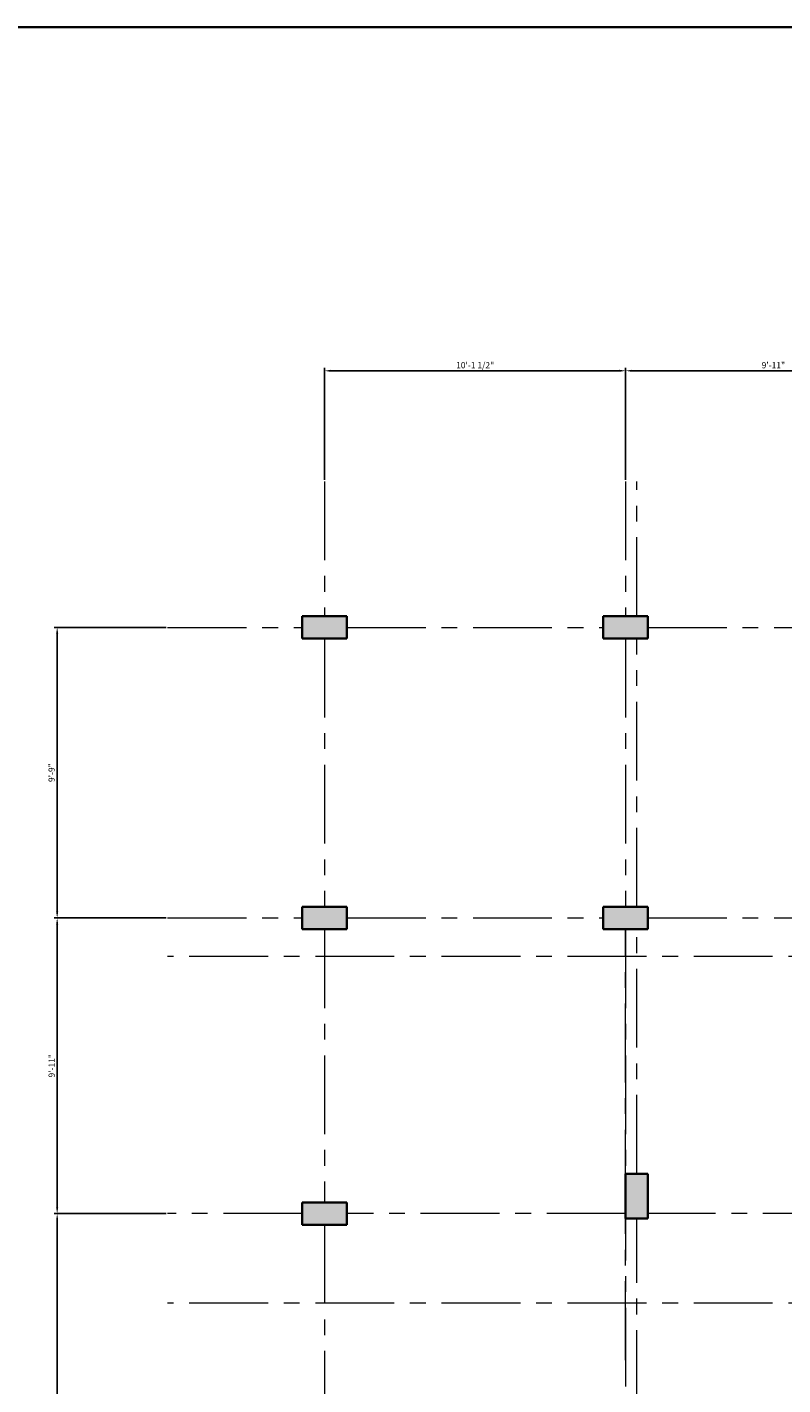
# Model space of a CAD drawing. Units: inches. Extents: x 2391 to 16591, y 7259 to 10239.
# Tile 24 of 27: x 3545 to 3850, y 9693 to 10239. Entities that reach past the tile are written whole.
import ezdxf

# ---------------------------------------------------------------- set-up
doc = ezdxf.new("R2010")
doc.units = ezdxf.units.IN
doc.linetypes.add('CENTER', pattern=[50.8, 31.75, -6.35, 6.35, -6.35])
for name, color, linetype, lineweight in [('A-ANNO-DIMS', 4, 'Continuous', 18), ('A-ANNO-TTLB', 7, 'Continuous', 35), ('A-COLS', 3, 'Continuous', 35), ('A-COLS-PATT', 3, 'Continuous', 13), ('A-GRID', 1, 'CENTER', 13)]:
    doc.layers.add(name, color=color, linetype=linetype, lineweight=lineweight)
doc.styles.get("Standard").update_dxf_attribs({"font": 'arial.ttf'})
doc.dimstyles.new('ISO-25', dxfattribs={"dimtxt": 2.5, "dimasz": 2.5, "dimexe": 1.25, "dimexo": 0.625, "dimtad": 1, "dimdec": 0, "dimlunit": 3, "dimtxsty": 'Standard', "dimcen": 2.5, "dimadec": 0, "dimazin": 0, "dimtfac": 1, "dimtdec": 0, "dimtmove": 0, "dimatfit": 3, "dimfxl": 1, "dimarcsym": 0})

# ---------------------------------------------------------------- blocks, each defined once
blk = doc.blocks.new('*D104')
at = {"layer": 'A-ANNO-DIMS', "color": 0, "lineweight": -2, "transparency": 16777216}
for p, q in [((3665.26, 10057.17), (3665.26, 10102.29)), ((3667.76, 10101.04), (3784.01, 10101.04)), ((3786.51, 10057.17), (3786.51, 10102.29))]:
    blk.add_line(p, q, dxfattribs=at)
at = {"layer": 'A-ANNO-DIMS', "color": 0, "transparency": 16777216}
for points in [[(3667.76, 10101.46), (3667.76, 10100.63), (3665.26, 10101.04)], [(3784.01, 10101.46), (3784.01, 10100.63), (3786.51, 10101.04)]]:
    blk.add_solid(points, dxfattribs=at)
at = {"layer": 'Defpoints', "color": 0, "transparency": 16777216}
for p in [(3786.51, 10101.04), (3665.26, 10056.54), (3786.51, 10056.54)]:
    blk.add_point(p, dxfattribs=at)
at = {"layer": 'A-ANNO-DIMS', "color": 0, "transparency": 16777216, "insert": (3725.89, 10102.96), "char_height": 2.5, "attachment_point": 5}
blk.add_mtext('10\'-1 1/2"', dxfattribs=at)
blk = doc.blocks.new('*D105')
at = {"layer": 'A-ANNO-DIMS', "color": 0, "lineweight": -2, "transparency": 16777216}
for p, q in [((3786.51, 10057.17), (3786.51, 10102.29)), ((3789.01, 10101.04), (3903.01, 10101.04)), ((3905.51, 10057.17), (3905.51, 10102.29))]:
    blk.add_line(p, q, dxfattribs=at)
at = {"layer": 'A-ANNO-DIMS', "color": 0, "transparency": 16777216}
for points in [[(3789.01, 10101.46), (3789.01, 10100.63), (3786.51, 10101.04)], [(3903.01, 10101.46), (3903.01, 10100.63), (3905.51, 10101.04)]]:
    blk.add_solid(points, dxfattribs=at)
at = {"layer": 'Defpoints', "color": 0, "transparency": 16777216}
for p in [(3905.51, 10101.04), (3786.51, 10056.54), (3905.51, 10056.54)]:
    blk.add_point(p, dxfattribs=at)
at = {"layer": 'A-ANNO-DIMS', "color": 0, "transparency": 16777216, "insert": (3846.01, 10102.95), "char_height": 2.5, "attachment_point": 5}
blk.add_mtext('9\'-11"', dxfattribs=at)
blk = doc.blocks.new('*D109')
at = {"layer": 'A-ANNO-DIMS', "color": 0, "lineweight": -2, "transparency": 16777216}
for p, q in [((3601.45, 9761.76), (3556.32, 9761.76)), ((3557.57, 9600.26), (3557.57, 9759.26)), ((3601.45, 9597.76), (3556.32, 9597.76))]:
    blk.add_line(p, q, dxfattribs=at)
at = {"layer": 'A-ANNO-DIMS', "color": 0, "transparency": 16777216}
for points in [[(3557.15, 9759.26), (3557.99, 9759.26), (3557.57, 9761.76)], [(3557.15, 9600.26), (3557.99, 9600.26), (3557.57, 9597.76)]]:
    blk.add_solid(points, dxfattribs=at)
at = {"layer": 'Defpoints', "color": 0, "transparency": 16777216}
for p in [(3557.57, 9761.76), (3602.07, 9761.76), (3602.07, 9597.76)]:
    blk.add_point(p, dxfattribs=at)
at = {"layer": 'A-ANNO-DIMS', "color": 0, "transparency": 16777216, "insert": (3555.67, 9679.76), "char_height": 2.5, "attachment_point": 5, "rotation": 90}
blk.add_mtext('13\'-8"', dxfattribs=at)
blk = doc.blocks.new('*D110')
at = {"layer": 'A-ANNO-DIMS', "color": 0, "lineweight": -2, "transparency": 16777216}
for p, q in [((3601.45, 9880.76), (3556.32, 9880.76)), ((3557.57, 9764.26), (3557.57, 9878.26)), ((3601.45, 9761.76), (3556.32, 9761.76))]:
    blk.add_line(p, q, dxfattribs=at)
at = {"layer": 'A-ANNO-DIMS', "color": 0, "transparency": 16777216}
for points in [[(3557.15, 9878.26), (3557.99, 9878.26), (3557.57, 9880.76)], [(3557.15, 9764.26), (3557.99, 9764.26), (3557.57, 9761.76)]]:
    blk.add_solid(points, dxfattribs=at)
at = {"layer": 'Defpoints', "color": 0, "transparency": 16777216}
for p in [(3557.57, 9880.76), (3602.07, 9880.76), (3602.07, 9761.76)]:
    blk.add_point(p, dxfattribs=at)
at = {"layer": 'A-ANNO-DIMS', "color": 0, "transparency": 16777216, "insert": (3555.67, 9821.26), "char_height": 2.5, "attachment_point": 5, "rotation": 90}
blk.add_mtext('9\'-11"', dxfattribs=at)
blk = doc.blocks.new('*D111')
at = {"layer": 'A-ANNO-DIMS', "color": 0, "lineweight": -2, "transparency": 16777216}
for p, q in [((3601.45, 9997.76), (3556.32, 9997.76)), ((3557.57, 9883.26), (3557.57, 9995.26)), ((3601.45, 9880.76), (3556.32, 9880.76))]:
    blk.add_line(p, q, dxfattribs=at)
at = {"layer": 'A-ANNO-DIMS', "color": 0, "transparency": 16777216}
for points in [[(3557.15, 9995.26), (3557.99, 9995.26), (3557.57, 9997.76)], [(3557.15, 9883.26), (3557.99, 9883.26), (3557.57, 9880.76)]]:
    blk.add_solid(points, dxfattribs=at)
at = {"layer": 'Defpoints', "color": 0, "transparency": 16777216}
for p in [(3557.57, 9997.76), (3602.07, 9997.76), (3602.07, 9880.76)]:
    blk.add_point(p, dxfattribs=at)
at = {"layer": 'A-ANNO-DIMS', "color": 0, "transparency": 16777216, "insert": (3555.67, 9939.26), "char_height": 2.5, "attachment_point": 5, "rotation": 90}
blk.add_mtext('9\'-9"', dxfattribs=at)

msp = doc.modelspace()

# ---------------------------------------------------------------- hatches: boundary and pattern name
at = {"layer": 'A-COLS-PATT'}
h = msp.add_hatch(color=256, dxfattribs=at)
h.dxf.hatch_style = 1
h.paths.add_polyline_path([(3674.26, 9993.26), (3674.26, 10002.26), (3656.26, 10002.26), (3656.26, 9993.26)])
h.paths.add_polyline_path([(3777.51, 10002.26), (3777.51, 9993.26), (3795.51, 9993.26), (3795.51, 10002.26)])
h.paths.add_polyline_path([(3896.51, 10002.26), (3896.51, 9993.26), (3914.51, 9993.26), (3914.51, 10002.26)])
h.paths.add_polyline_path([(3999.01, 10002.26), (3999.01, 9993.26), (4017.01, 9993.26), (4017.01, 10002.26)])
h.paths.add_polyline_path([(4017.01, 9860.76), (4017.01, 9869.76), (3999.01, 9869.76), (3999.01, 9860.76)])
h.paths.add_polyline_path([(3914.51, 9860.76), (3914.51, 9869.76), (3896.51, 9869.76), (3896.51, 9860.76)])
h.paths.add_polyline_path([(3777.51, 9885.26), (3777.51, 9876.26), (3795.51, 9876.26), (3795.51, 9885.26)])
h.paths.add_polyline_path([(3674.26, 9876.26), (3674.26, 9885.26), (3656.26, 9885.26), (3656.26, 9876.26)])
h.paths.add_polyline_path([(3656.26, 9766.26), (3656.26, 9757.26), (3674.26, 9757.26), (3674.26, 9766.26)])
h.paths.add_polyline_path([(3786.51, 9759.76), (3795.51, 9759.76), (3795.51, 9777.76), (3786.51, 9777.76)])
h.paths.add_polyline_path([(3914.51, 9721.26), (3914.51, 9730.26), (3896.51, 9730.26), (3896.51, 9721.26)])
h.paths.add_polyline_path([(3999.01, 9730.26), (3999.01, 9721.26), (4017.01, 9721.26), (4017.01, 9730.26)])
h.paths.add_polyline_path([(4017.01, 9632.26), (4017.01, 9641.26), (3999.01, 9641.26), (3999.01, 9632.26)])
h.paths.add_polyline_path([(3914.51, 9632.26), (3914.51, 9641.26), (3896.51, 9641.26), (3896.51, 9632.26)])
h.paths.add_polyline_path([(3795.51, 9632.26), (3786.51, 9632.26), (3786.51, 9614.26), (3795.51, 9614.26)])
h.paths.add_polyline_path([(3656.26, 9602.26), (3656.26, 9593.26), (3674.26, 9593.26), (3674.26, 9602.26)])
h.paths.add_polyline_path([(3674.26, 9471.26), (3674.26, 9480.26), (3656.26, 9480.26), (3656.26, 9471.26)])
h.paths.add_polyline_path([(3795.51, 9489.26), (3786.51, 9489.26), (3786.51, 9471.26), (3795.51, 9471.26)])
h.paths.add_polyline_path([(3896.51, 9502.76), (3896.51, 9493.76), (3914.51, 9493.76), (3914.51, 9502.76)])
h.paths.add_polyline_path([(3999.01, 9502.76), (3999.01, 9493.76), (4017.01, 9493.76), (4017.01, 9502.76)])
h.paths.add_polyline_path([(4017.01, 9354.26), (4017.01, 9363.26), (3999.01, 9363.26), (3999.01, 9354.26)])
h.paths.add_polyline_path([(3914.51, 9354.26), (3914.51, 9363.26), (3896.51, 9363.26), (3896.51, 9354.26)])
h.paths.add_polyline_path([(3795.51, 9354.26), (3795.51, 9363.26), (3777.51, 9363.26), (3777.51, 9354.26)])
h.paths.add_polyline_path([(3674.26, 9354.26), (3674.26, 9363.26), (3656.26, 9363.26), (3656.26, 9354.26)])

# ---------------------------------------------------------------- linework, layer by layer
at = {"layer": 'A-ANNO-TTLB'}
msp.add_lwpolyline([(2391.28, 10239.38), (4154.2, 10239.38), (4154.2, 7258.54), (2391.28, 7258.54)], close=True, dxfattribs=at)
at = {"layer": 'A-COLS'}
for p, q in [((3656.26, 10002.26), (3674.26, 10002.26)), ((3656.26, 9993.26), (3656.26, 10002.26)), ((3674.26, 10002.26), (3674.26, 9993.26)), ((3777.51, 10002.26), (3795.51, 10002.26)), ((3777.51, 9993.26), (3777.51, 10002.26)), ((3795.51, 10002.26), (3795.51, 9993.26)), ((3674.26, 9993.26), (3656.26, 9993.26)), ((3795.51, 9993.26), (3777.51, 9993.26)), ((3656.26, 9885.26), (3674.26, 9885.26)), ((3656.26, 9876.26), (3656.26, 9885.26)), ((3674.26, 9885.26), (3674.26, 9876.26)), ((3777.51, 9885.26), (3795.51, 9885.26)), ((3777.51, 9876.26), (3777.51, 9885.26)), ((3795.51, 9885.26), (3795.51, 9876.26)), ((3674.26, 9876.26), (3656.26, 9876.26)), ((3795.51, 9876.26), (3777.51, 9876.26)), ((3786.51, 9759.76), (3786.51, 9777.76)), ((3786.51, 9777.76), (3795.51, 9777.76)), ((3795.51, 9777.76), (3795.51, 9759.76)), ((3656.26, 9766.26), (3674.26, 9766.26)), ((3656.26, 9757.26), (3656.26, 9766.26)), ((3674.26, 9766.26), (3674.26, 9757.26)), ((3674.26, 9757.26), (3656.26, 9757.26)), ((3795.51, 9759.76), (3786.51, 9759.76))]:
    msp.add_line(p, q, dxfattribs=at)
at = {"layer": 'A-GRID'}
for p, q in [((3665.26, 10056.54), (3665.26, 10002.26)), ((3786.51, 10056.54), (3786.51, 10002.26)), ((3791.01, 10002.26), (3791.01, 10056.54)), ((3602.07, 9997.76), (3656.26, 9997.76)), ((3674.26, 9997.76), (3777.51, 9997.76)), ((3795.51, 9997.76), (3896.51, 9997.76)), ((3665.26, 9993.26), (3665.26, 9885.26)), ((3786.51, 9993.26), (3786.51, 9885.26)), ((3791.01, 9885.26), (3791.01, 9993.26)), ((3602.07, 9880.76), (3656.26, 9880.76)), ((3674.26, 9880.76), (3777.51, 9880.76)), ((3795.51, 9880.76), (4076.77, 9880.76)), ((3665.26, 9876.26), (3665.26, 9766.26)), ((3786.51, 9763.76), (3786.51, 9876.26)), ((3786.51, 9876.26), (3786.51, 9363.26)), ((3791.01, 9777.76), (3791.01, 9876.26)), ((3896.51, 9865.26), (3602.07, 9865.26)), ((3656.26, 9761.76), (3602.07, 9761.76)), ((3786.51, 9761.76), (3674.26, 9761.76)), ((4076.77, 9761.76), (3795.51, 9761.76)), ((3665.26, 9757.26), (3665.26, 9602.26)), ((3786.51, 9702.76), (3786.51, 9759.76)), ((3791.01, 9632.26), (3791.01, 9759.76)), ((3896.51, 9725.76), (3602.07, 9725.76))]:
    msp.add_line(p, q, dxfattribs=at)

# ---------------------------------------------------------------- dimensions: what is measured, and where the dimension line sits
at = {"layer": 'A-ANNO-DIMS'}
for base, p1, p2, picture, middle in [((3786.51174, 10101.044733), (3665.26174, 10056.544733), (3786.51174, 10056.544733), '*D104', (3725.88674, 10102.96236602)), ((3905.51, 10101.04), (3786.51, 10056.54), (3905.51, 10056.54), '*D105', (3846.01, 10102.95))]:
    dim = msp.add_linear_dim(base=base, p1=p1, p2=p2, dimstyle='ISO-25', override={"dimdec": 1, "dimlfac": 1, "dimrnd": 0, "dimzin": 1, "dimdsep": 46, "dimlunit": 4, "dimfrac": 2}, dxfattribs=at)
    dim.commit()
    dim.dimension.update_dxf_attribs({"geometry": picture, "text_midpoint": middle})
for base, p1, p2, picture, middle in [((3557.57, 9997.76), (3602.07, 9880.76), (3602.07, 9997.76), '*D111', (3555.67, 9939.26)), ((3557.57, 9880.76), (3602.07, 9761.76), (3602.07, 9880.76), '*D110', (3555.67, 9821.26)), ((3557.57, 9761.76), (3602.07, 9597.76), (3602.07, 9761.76), '*D109', (3555.67, 9679.76))]:
    dim = msp.add_linear_dim(base=base, p1=p1, p2=p2, angle=90, dimstyle='ISO-25', override={"dimdec": 1, "dimlfac": 1, "dimrnd": 0, "dimzin": 1, "dimdsep": 46, "dimlunit": 4, "dimfrac": 2}, dxfattribs=at)
    dim.commit()
    dim.dimension.update_dxf_attribs({"geometry": picture, "text_midpoint": middle})

doc.saveas('drawing.dxf')
